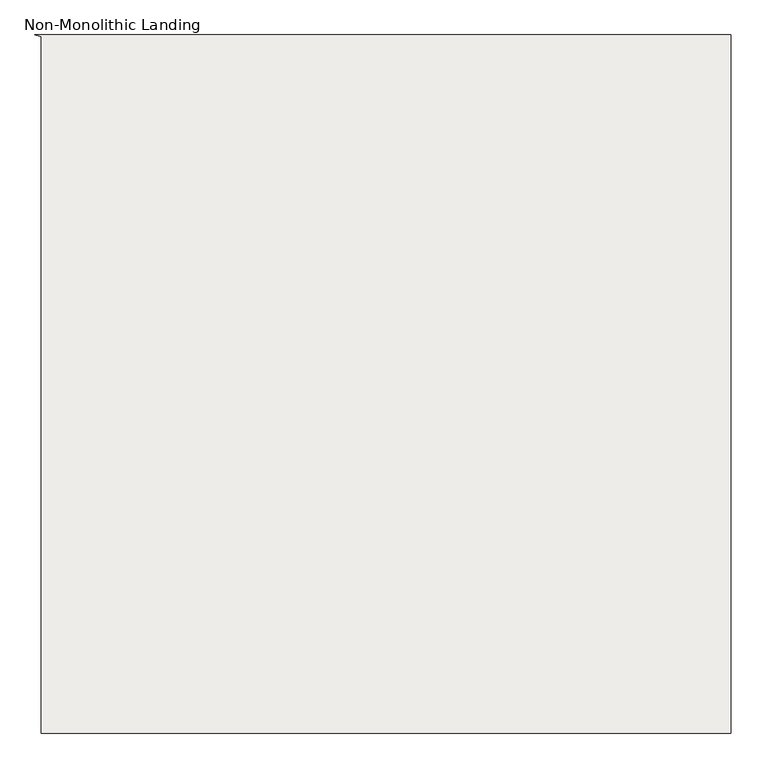
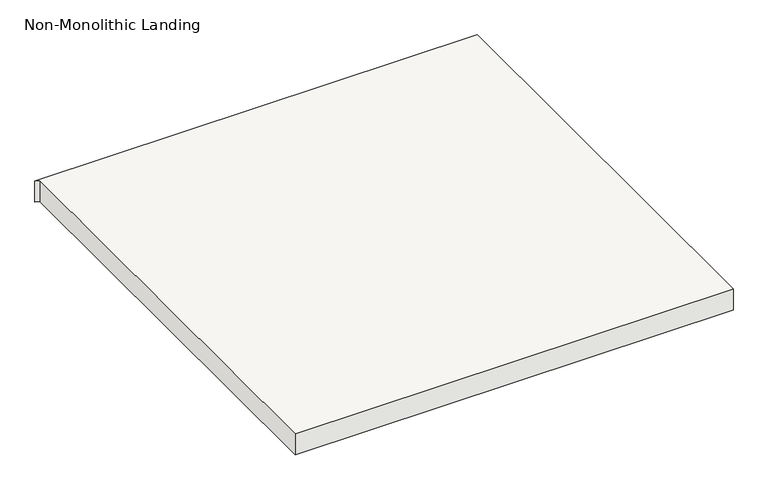
"""IFC4 building model written with IfcOpenShell, lengths in millimetres: slab geometry, Non-Monolithic Landing."""

from ifc_helpers import new_model, si_unit, frame, origin, place, context, project, spatial, polyline, outline, extrude, source, transform, mapped, element, save


def non_monolithic_landing_62522cc9(model_context):
    return source(origin(), model_context, "Body", "SweptSolid", [
        extrude(outline(polyline([(-9477.5794909, -3248.5618509), (-9477.5794909, -4251.1618509), (-10468.1794909, -4251.1618509), (-10468.1794909, -3251.1360696), (-10477.6052721, -3248.5618509), (-9477.5794909, -3248.5618509)])), frame((0.0, 0.0, 11622.0470588), z_axis=(0.0, 0.0, 1.0), x_axis=(1.0, 0.0, 0.0)), (0.0, 0.0, 1.0), 50.0),
    ])


if __name__ == "__main__":
    model = new_model("IFC4")
    model_context = context("Model", 3, world=origin())
    ifc_project = project(units=[si_unit("LENGTHUNIT", "METRE", prefix="MILLI")], contexts=[model_context])
    site = spatial("IfcSite", under=ifc_project)
    building = spatial("IfcBuilding", under=site)
    placement = place(None, origin())
    non_monolithic_landing_shape = non_monolithic_landing_62522cc9(model_context)
    element("IfcSlab", 1, ObjectType="Non-Monolithic Landing", at=placement, inside=building, context=model_context, shape_type="MappedRepresentation", body=[
        mapped(non_monolithic_landing_shape, transform((0.0, 0.0, 0.0), x_axis=(1.0, 0.0, 0.0), y_axis=(0.0, 1.0, 0.0), z_axis=(0.0, 0.0, 1.0))),
    ])
    save(model, "model.ifc")
